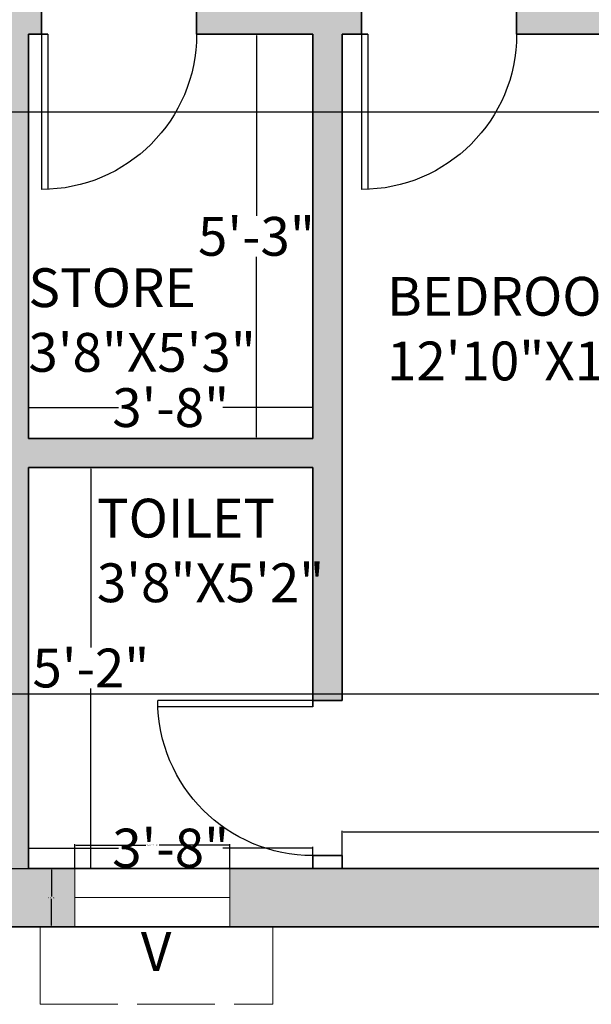
# Model space of a CAD drawing. Units: inches. Extents: x -5 to 482, y -460 to 66.
# Tile 14 of 31: x 218 to 306, y -434 to -282. Entities that reach past the tile are written whole.
import ezdxf

# ---------------------------------------------------------------- set-up
doc = ezdxf.new("R2010")
doc.units = ezdxf.units.IN
doc.header["$MEASUREMENT"] = 0
doc.linetypes.add('ACAD_ISO02W100', pattern=[15, 12, -3])
for name, color, linetype, lineweight in [('A-ANNO-DIMS', 2, 'Continuous', 18), ('A-ANNO-TEXT', 7, 'Continuous', 18), ('A-AREA-IDEN', 7, 'Continuous', 18), ('A-DOOR', 3, 'Continuous', 25), ('A-GLAZ', 4, 'Continuous', 18), ('A-GLAZ-OVHD', 4, 'ACAD_ISO02W100', 13), ('A-WALL', 7, 'Continuous', 35), ('A-WALL-PATT', 152, 'Continuous', 13)]:
    doc.layers.add(name, color=color, linetype=linetype, lineweight=lineweight)
doc.styles.get("Standard").update_dxf_attribs({"font": 'arial.ttf'})
doc.dimstyles.get("Standard").update_dxf_attribs({"dimtxt": 0.18, "dimasz": 0.18, "dimexe": 0.18, "dimexo": 0.0625, "dimgap": 0.09, "dimtad": 0, "dimtih": 1, "dimtoh": 1, "dimdec": 0, "dimzin": 0, "dimdsep": 46, "dimlunit": 3, "dimtxsty": 'Standard', "dimcen": 0.09, "dimadec": 0, "dimazin": 0, "dimtfac": 1, "dimtdec": 0, "dimtofl": 0, "dimtmove": 0, "dimatfit": 3, "dimfxl": 1, "dimtolj": 1, "dimtzin": 0, "dimarcsym": 0})

# ---------------------------------------------------------------- blocks, each defined once
blk = doc.blocks.new('*D23')
at = {"layer": 'A-ANNO-DIMS', "color": 0, "lineweight": -2, "transparency": 16777216}
for p, q in [((255.46, -283.85), (253.96, -283.85)), ((254.14, -284.03), (254.14, -311.94)), ((254.14, -346.17), (254.14, -318.25)), ((255.46, -346.35), (253.96, -346.35))]:
    blk.add_line(p, q, dxfattribs=at)
at = {"layer": 'A-ANNO-DIMS', "color": 0, "transparency": 16777216}
for points in [[(254.11, -284.03), (254.17, -284.03), (254.14, -283.85)], [(254.11, -346.17), (254.17, -346.17), (254.14, -346.35)]]:
    blk.add_solid(points, dxfattribs=at)
at = {"layer": 'Defpoints', "color": 0, "transparency": 16777216}
for p in [(254.14, -283.85), (255.52, -283.85), (255.52, -346.35)]:
    blk.add_point(p, dxfattribs=at)
at = {"layer": 'A-ANNO-DIMS', "color": 0, "transparency": 16777216, "insert": (254.14, -315.1), "char_height": 6, "attachment_point": 5}
blk.add_mtext('\\A1;5\'-3"', dxfattribs=at)
blk = doc.blocks.new('*D24')
at = {"layer": 'A-ANNO-DIMS', "color": 0, "lineweight": -2, "transparency": 16777216}
for p, q in [((218.88, -341.52), (218.88, -341.4)), ((219.06, -341.58), (232.81, -341.58)), ((262.7, -341.58), (248.94, -341.58)), ((262.88, -341.52), (262.88, -341.4))]:
    blk.add_line(p, q, dxfattribs=at)
at = {"layer": 'A-ANNO-DIMS', "color": 0, "transparency": 16777216}
for points in [[(219.06, -341.55), (219.06, -341.61), (218.88, -341.58)], [(262.7, -341.55), (262.7, -341.61), (262.88, -341.58)]]:
    blk.add_solid(points, dxfattribs=at)
at = {"layer": 'Defpoints', "color": 0, "transparency": 16777216}
for p in [(218.88, -341.58), (262.88, -341.58), (262.88, -341.58)]:
    blk.add_point(p, dxfattribs=at)
at = {"layer": 'A-ANNO-DIMS', "color": 0, "transparency": 16777216, "insert": (240.88, -341.58), "char_height": 6, "attachment_point": 5}
blk.add_mtext('\\A1;3\'-8"', dxfattribs=at)
blk = doc.blocks.new('*D25')
at = {"layer": 'A-ANNO-DIMS', "color": 0, "lineweight": -2, "transparency": 16777216}
for p, q in [((228.54, -351.03), (228.54, -378.7)), ((228.6, -350.85), (228.72, -350.85)), ((228.54, -412.67), (228.54, -385)), ((226.12, -412.85), (228.72, -412.85))]:
    blk.add_line(p, q, dxfattribs=at)
at = {"layer": 'A-ANNO-DIMS', "color": 0, "transparency": 16777216}
for points in [[(228.51, -351.03), (228.57, -351.03), (228.54, -350.85)], [(228.51, -412.67), (228.57, -412.67), (228.54, -412.85)]]:
    blk.add_solid(points, dxfattribs=at)
at = {"layer": 'Defpoints', "color": 0, "transparency": 16777216}
for p in [(228.54, -350.85), (228.54, -350.85), (226.05, -412.85)]:
    blk.add_point(p, dxfattribs=at)
at = {"layer": 'A-ANNO-DIMS', "color": 0, "transparency": 16777216, "insert": (228.54, -381.85), "char_height": 6, "attachment_point": 5}
blk.add_mtext('\\A1;5\'-2"', dxfattribs=at)
blk = doc.blocks.new('*D26')
at = {"layer": 'A-ANNO-DIMS', "color": 0, "lineweight": -2, "transparency": 16777216}
for p, q in [((218.88, -410.79), (218.88, -409.51)), ((262.88, -410.79), (262.88, -409.51)), ((219.06, -409.69), (232.81, -409.69)), ((262.7, -409.69), (248.94, -409.69))]:
    blk.add_line(p, q, dxfattribs=at)
at = {"layer": 'A-ANNO-DIMS', "color": 0, "transparency": 16777216}
for points in [[(219.06, -409.66), (219.06, -409.72), (218.88, -409.69)], [(262.7, -409.66), (262.7, -409.72), (262.88, -409.69)]]:
    blk.add_solid(points, dxfattribs=at)
at = {"layer": 'Defpoints', "color": 0, "transparency": 16777216}
for p in [(218.88, -409.69), (218.88, -410.85), (262.88, -410.85)]:
    blk.add_point(p, dxfattribs=at)
at = {"layer": 'A-ANNO-DIMS', "color": 0, "transparency": 16777216, "insert": (240.88, -409.69), "char_height": 6, "attachment_point": 5}
blk.add_mtext('\\A1;3\'-8"', dxfattribs=at)
blk = doc.blocks.new('*D28')
at = {"layer": 'A-ANNO-DIMS', "color": 0, "lineweight": -2, "transparency": 16777216}
for p, q in [((267.38, -410.79), (267.38, -407)), ((267.56, -407.18), (331.93, -407.18)), ((421.2, -407.18), (356.82, -407.18)), ((421.38, -410.79), (421.38, -407))]:
    blk.add_line(p, q, dxfattribs=at)
at = {"layer": 'A-ANNO-DIMS', "color": 0, "transparency": 16777216}
for points in [[(267.56, -407.15), (267.56, -407.21), (267.38, -407.18)], [(421.2, -407.15), (421.2, -407.21), (421.38, -407.18)]]:
    blk.add_solid(points, dxfattribs=at)
at = {"layer": 'Defpoints', "color": 0, "transparency": 16777216}
for p in [(421.38, -407.18), (267.38, -410.85), (421.38, -410.85)]:
    blk.add_point(p, dxfattribs=at)
at = {"layer": 'A-ANNO-DIMS', "color": 0, "transparency": 16777216, "insert": (344.38, -407.18), "char_height": 6, "attachment_point": 5}
blk.add_mtext('\\A1;12\'-10"', dxfattribs=at)
blk = doc.blocks.new('DOOR-SWING-24IN')
for p, q in [((24, 1), (0, 1)), ((24, 0), (0, 0))]:
    blk.add_line(p, q)
blk.add_arc((24, 0), 24, 90, 180)
blk = doc.blocks.new('VENT-GLAZ-24IN')
for p, q in [((0, 9), (24, 9)), ((0, 4.5), (24, 4.5)), ((24, 0), (0, 0))]:
    blk.add_line(p, q)
blk = doc.blocks.new('VENT-SHADE-36IN')
for p, q in [((0, 0), (0, 12)), ((36, 0), (36, 12)), ((0, 0), (36, 0))]:
    blk.add_line(p, q)
blk = doc.blocks.new('*D49')
at = {"layer": 'A-ANNO-DIMS', "color": 0, "lineweight": -2, "transparency": 16777216}
for p, q in [((226.05, -412.79), (226.05, -409.07)), ((226.23, -409.25), (237.04, -409.25)), ((249.87, -409.25), (239.07, -409.25)), ((250.05, -412.79), (250.05, -409.07))]:
    blk.add_line(p, q, dxfattribs=at)
at = {"layer": 'A-ANNO-DIMS', "color": 0, "transparency": 16777216}
for points in [[(226.23, -409.22), (226.23, -409.28), (226.05, -409.25)], [(249.87, -409.22), (249.87, -409.28), (250.05, -409.25)]]:
    blk.add_solid(points, dxfattribs=at)
at = {"layer": 'Defpoints', "color": 0, "transparency": 16777216}
for p in [(250.05, -409.25), (226.05, -412.85), (250.05, -412.85)]:
    blk.add_point(p, dxfattribs=at)
at = {"layer": 'A-ANNO-DIMS', "color": 0, "transparency": 16777216, "insert": (238.05, -409.25), "char_height": 0.18, "attachment_point": 5}
blk.add_mtext('\\A1;VENT 2\'-0" TYP.', dxfattribs=at)
blk = doc.blocks.new('*D50')
at = {"layer": 'A-ANNO-DIMS', "color": 0, "lineweight": -2, "transparency": 16777216}
for p, q in [((225.99, -412.85), (222.27, -412.85)), ((222.45, -413.03), (222.45, -417.17)), ((222.45, -421.67), (222.45, -417.53)), ((225.99, -421.85), (222.27, -421.85))]:
    blk.add_line(p, q, dxfattribs=at)
at = {"layer": 'A-ANNO-DIMS', "color": 0, "transparency": 16777216}
for points in [[(222.42, -413.03), (222.48, -413.03), (222.45, -412.85)], [(222.42, -421.67), (222.48, -421.67), (222.45, -421.85)]]:
    blk.add_solid(points, dxfattribs=at)
at = {"layer": 'Defpoints', "color": 0, "transparency": 16777216}
for p in [(222.45, -412.85), (226.05, -412.85), (226.05, -421.85)]:
    blk.add_point(p, dxfattribs=at)
at = {"layer": 'A-ANNO-DIMS', "color": 0, "transparency": 16777216, "insert": (222.45, -417.35), "char_height": 0.18, "attachment_point": 5}
blk.add_mtext('\\A1;0\'-9" TYP.', dxfattribs=at)
blk = doc.blocks.new('*D74')
at = {"layer": 'A-ANNO-DIMS', "color": 0, "lineweight": -2, "transparency": 16777216}
for p, q in [((214.44, -295.86), (468.16, -295.86)), ((467.98, -296.04), (467.98, -340.68)), ((467.98, -385.68), (467.98, -341.04)), ((214.44, -385.86), (468.16, -385.86))]:
    blk.add_line(p, q, dxfattribs=at)
at = {"layer": 'A-ANNO-DIMS', "color": 0, "transparency": 16777216}
for points in [[(467.95, -296.04), (468.01, -296.04), (467.98, -295.86)], [(467.95, -385.68), (468.01, -385.68), (467.98, -385.86)]]:
    blk.add_solid(points, dxfattribs=at)
at = {"layer": 'Defpoints', "color": 0, "transparency": 16777216}
for p in [(214.38, -295.86), (467.98, -295.86), (214.38, -385.86)]:
    blk.add_point(p, dxfattribs=at)
at = {"layer": 'A-ANNO-DIMS', "color": 0, "transparency": 16777216, "insert": (467.98, -340.86), "char_height": 0.18, "attachment_point": 5}
blk.add_mtext('\\A1;7\'-6"', dxfattribs=at)
blk = doc.blocks.new('*D75')
at = {"layer": 'A-ANNO-DIMS', "color": 0, "lineweight": -2, "transparency": 16777216}
for p, q in [((214.44, -385.86), (468.16, -385.86)), ((467.98, -386.04), (467.98, -399.17)), ((467.98, -412.67), (467.98, -399.54)), ((214.44, -412.85), (468.16, -412.85))]:
    blk.add_line(p, q, dxfattribs=at)
at = {"layer": 'A-ANNO-DIMS', "color": 0, "transparency": 16777216}
for points in [[(467.95, -386.04), (468.01, -386.04), (467.98, -385.86)], [(467.95, -412.67), (468.01, -412.67), (467.98, -412.85)]]:
    blk.add_solid(points, dxfattribs=at)
at = {"layer": 'Defpoints', "color": 0, "transparency": 16777216}
for p in [(214.38, -385.86), (467.98, -385.86), (214.38, -412.85)]:
    blk.add_point(p, dxfattribs=at)
at = {"layer": 'A-ANNO-DIMS', "color": 0, "transparency": 16777216, "insert": (467.98, -399.35), "char_height": 0.18, "attachment_point": 5}
blk.add_mtext('\\A1;2\'-3"', dxfattribs=at)

msp = doc.modelspace()

# ---------------------------------------------------------------- hatches: boundary and pattern name
at = {"layer": 'A-WALL-PATT'}
h = msp.add_hatch(color=256, dxfattribs=at)
h.dxf.hatch_style = 1
h.paths.add_polyline_path([(149.38, -412.85), (144.38, -412.85), (144.38, -283.85), (144.38, -279.35), (133.88, -279.35), (133.88, -283.85), (139.88, -283.85), (139.88, -412.85), (133.51, -412.85), (133.51, -413.92), (102.65, -413.92), (102.65, -421.02), (133.51, -421.02), (133.51, -421.85), (149.38, -421.85)])
h.paths.add_polyline_path([(226.05, -412.85), (218.88, -412.85), (218.88, -350.85), (262.88, -350.85), (262.88, -386.85), (267.38, -386.85), (267.38, -283.85), (270.38, -283.85), (270.38, -279.35), (244.88, -279.35), (244.88, -283.85), (262.88, -283.85), (262.88, -346.35), (218.88, -346.35), (218.88, -283.85), (220.88, -283.85), (220.88, -279.35), (214.38, -279.35), (214.38, -283.85), (214.38, -412.85), (209.38, -412.85), (209.38, -421.85), (226.05, -421.85)])
h.paths.add_polyline_path([(315.81, -412.85), (250.05, -412.85), (250.05, -421.85), (315.81, -421.85)])
h.paths.add_polyline_path([(430.38, -378.35), (421.38, -378.35), (421.38, -412.85), (375.81, -412.85), (375.81, -421.85), (430.38, -421.85)])
h.paths.add_polyline_path([(78.69, -413.92), (47.68, -413.92), (47.68, -412.85), (41.88, -412.85), (41.88, -283.85), (109.88, -283.85), (109.88, -279.35), (41.88, -279.35), (41.88, -241.85), (32.88, -241.85), (32.88, -421.85), (47.68, -421.85), (47.68, -421.02), (78.69, -421.02)])
h.paths.add_polyline_path([(41.88, -144.35), (154.38, -144.35), (154.38, -137.85), (149.88, -137.85), (149.88, -139.85), (41.88, -139.85), (41.88, -97.85), (32.88, -97.85), (32.88, -181.85), (41.88, -181.85)])
h.paths.add_polyline_path([(430.38, -241.85), (421.38, -241.85), (421.38, -279.35), (309.38, -279.35), (309.38, -170.35), (304.88, -170.35), (304.88, -279.35), (294.38, -279.35), (294.38, -283.85), (421.38, -283.85), (421.38, -318.35), (430.38, -318.35)])
h.paths.add_polyline_path([(430.38, -119.85), (421.38, -119.85), (421.38, -139.85), (419.38, -139.85), (419.38, -144.35), (421.38, -144.35), (421.38, -181.85), (430.38, -181.85)])
h.paths.add_polyline_path([(395.38, -139.85), (377.38, -139.85), (377.38, -75.85), (421.38, -75.85), (421.38, -95.85), (430.38, -95.85), (430.38, -45.6), (421.38, -45.6), (421.38, -71.35), (377.38, -71.35), (377.38, -22.85), (372.88, -22.85), (372.88, -139.85), (242.88, -139.85), (242.88, -137.85), (238.38, -137.85), (238.38, -144.35), (304.88, -144.35), (304.88, -146.35), (309.38, -146.35), (309.38, -144.35), (395.38, -144.35)])
h.paths.add_polyline_path([(65.88, 13.15), (32.88, 13.15), (32.88, -37.85), (41.88, -37.85), (41.88, 4.15), (65.88, 4.15)])
h.paths.add_polyline_path([(166.38, 13.15), (125.88, 13.15), (125.88, 4.15), (149.88, 4.15), (149.88, -113.85), (154.38, -113.85), (154.38, 4.15), (166.38, 4.15)])
h.paths.add_polyline_path([(277.88, 13.15), (226.38, 13.15), (226.38, 4.15), (238.38, 4.15), (238.38, -113.85), (242.88, -113.85), (242.88, 4.15), (277.88, 4.15)])
h.paths.add_polyline_path([(430.38, 13.15), (337.88, 13.15), (337.88, 4.15), (372.88, 4.15), (372.88, 1.15), (377.38, 1.15), (377.38, 4.15), (421.38, 4.15), (421.38, -21.6), (430.38, -21.6)])

# ---------------------------------------------------------------- linework, layer by layer
at = {"layer": 'A-GLAZ'}
for p, q in [((226.05, -421.85), (226.05, -412.85)), ((250.05, -412.85), (250.05, -421.85))]:
    msp.add_line(p, q, dxfattribs=at)
at = {"layer": 'A-GLAZ-OVHD'}
msp.add_line((220.68, -433.85), (220.68, -433.85), dxfattribs=at)
at = {"layer": 'A-WALL'}
for p, q in [((220.88, -283.85), (220.88, -279.35)), ((244.88, -283.85), (244.88, -279.35)), ((270.38, -283.85), (270.38, -279.35)), ((294.38, -279.35), (294.38, -283.85)), ((218.88, -283.85), (218.88, -346.35)), ((218.88, -283.85), (221.88, -283.85)), ((244.88, -283.85), (262.88, -283.85)), ((262.88, -283.85), (262.88, -346.35)), ((267.38, -283.85), (267.38, -386.85)), ((267.38, -283.85), (271.38, -283.85)), ((294.38, -283.85), (421.38, -283.85)), ((218.88, -346.35), (262.88, -346.35)), ((218.88, -350.85), (262.88, -350.85)), ((218.88, -350.85), (218.88, -412.85)), ((262.88, -350.85), (262.88, -387.85)), ((267.38, -386.85), (262.88, -386.85)), ((262.88, -410.85), (267.38, -410.85)), ((262.88, -410.85), (262.88, -412.85)), ((267.38, -410.85), (267.38, -412.85)), ((218.88, -412.85), (421.38, -412.85)), ((133.51, -421.85), (430.38, -421.85))]:
    msp.add_line(p, q, dxfattribs=at)

# ---------------------------------------------------------------- block references
at = {"layer": 'A-DOOR', "extrusion": (0, 0, -1), "zscale": -1}
for p, rotation in [((-220.88, -307.85), 89.99999999999991), ((-270.38, -307.85), 89.99999999999991), ((-238.88, -386.85), 180)]:
    msp.add_blockref('DOOR-SWING-24IN', p, dxfattribs=dict(at, rotation=rotation))
at = {"layer": 'A-GLAZ'}
msp.add_blockref('VENT-GLAZ-24IN', (226.05, -421.85), dxfattribs=at)
at = {"layer": 'A-GLAZ-OVHD'}
msp.add_blockref('VENT-SHADE-36IN', (220.68, -433.85), dxfattribs=at)

# ---------------------------------------------------------------- texts
at = {"layer": 'A-ANNO-TEXT', "insert": (236.27, -422.69), "char_height": 6, "attachment_point": 1}
msp.add_mtext('V', dxfattribs=at)
at = {"layer": 'A-AREA-IDEN', "char_height": 6, "attachment_point": 1}
for s, insert in [('STORE\\P3\'8"X5\'3"', (218.88, -320.04)), ('BEDROOM\\P12\'10"X10\'9"', (274.34, -321.37)), ('TOILET\\P3\'8"X5\'2"', (229.47, -355.67))]:
    msp.add_mtext(s, dxfattribs=dict(at, insert=insert))

# ---------------------------------------------------------------- dimensions: what is measured, and where the dimension line sits
at = {"layer": 'A-ANNO-DIMS'}
for base, p1, p2, override, picture, middle in [((254.14428543, -283.84866403), (255.52032836, -346.34866403), (255.52032836, -283.84866403), {"dimtxt": 6, "dimclrd": 0, "dimclre": 0, "dimclrt": 0}, '*D23', (254.14428543, -315.09866403)), ((467.98, -295.86), (214.38, -385.86), (214.38, -295.86), {"dimdec": 1, "dimlfac": 1, "dimrnd": 0, "dimzin": 1, "dimdsep": 46, "dimlunit": 4, "dimfrac": 2}, '*D74', (467.98, -340.86)), ((228.54, -350.85), (226.05, -412.85), (228.54, -350.85), {"dimtxt": 6, "dimclrd": 0, "dimclre": 0, "dimclrt": 0}, '*D25', (228.54, -381.85)), ((467.98, -385.86), (214.38, -412.85), (214.38, -385.86), {"dimdec": 1, "dimlfac": 1, "dimrnd": 0, "dimzin": 1, "dimdsep": 46, "dimlunit": 4, "dimfrac": 2}, '*D75', (467.98, -399.35))]:
    dim = msp.add_linear_dim(base=base, p1=p1, p2=p2, angle=90, dimstyle='Standard', override=override, dxfattribs=at)
    dim.commit()
    dim.dimension.update_dxf_attribs({"geometry": picture, "text_midpoint": middle})
for base, p1, p2, picture, middle in [((262.88, -341.58), (218.88, -341.58), (262.88, -341.58), '*D24', (240.88, -341.58)), ((421.38, -407.18), (267.38, -410.85), (421.38, -410.85), '*D28', (344.38, -407.18)), ((218.88, -409.69), (262.88, -410.85), (218.88, -410.85), '*D26', (240.88, -409.69))]:
    dim = msp.add_linear_dim(base=base, p1=p1, p2=p2, dimstyle='Standard', override={"dimtxt": 6, "dimclrd": 0, "dimclre": 0, "dimclrt": 0}, dxfattribs=at)
    dim.commit()
    dim.dimension.update_dxf_attribs({"geometry": picture, "text_midpoint": middle})
dim = msp.add_linear_dim(base=(250.05, -409.25), p1=(226.05, -412.85), p2=(250.05, -412.85), text='VENT <> TYP.', dimstyle='Standard', override={"dimdec": 1, "dimlfac": 1, "dimrnd": 0, "dimzin": 1, "dimdsep": 46, "dimlunit": 4, "dimfrac": 2}, dxfattribs=at)
dim.commit()
dim.dimension.update_dxf_attribs({"geometry": '*D49', "text_midpoint": (238.05, -409.25)})
dim = msp.add_linear_dim(base=(222.45, -412.85), p1=(226.05, -421.85), p2=(226.05, -412.85), angle=90, text='<> TYP.', dimstyle='Standard', override={"dimdec": 1, "dimlfac": 1, "dimrnd": 0, "dimzin": 1, "dimdsep": 46, "dimlunit": 4, "dimfrac": 2}, dxfattribs=at)
dim.commit()
dim.dimension.update_dxf_attribs({"geometry": '*D50', "text_midpoint": (222.45, -417.35)})

doc.saveas('drawing.dxf')
